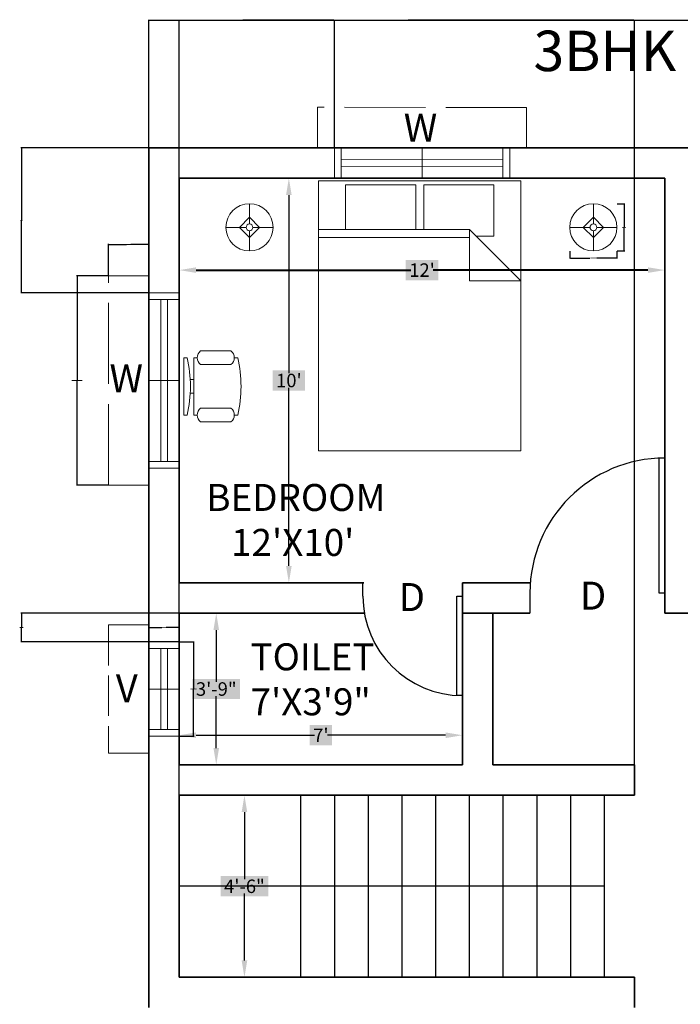
# Model space of a CAD drawing. Units: inches. Extents: x -128 to 854, y -395 to 398.
# Tile 35 of 61: x -88 to 107, y 95 to 387. Entities that reach past the tile are written whole.
import ezdxf

# ---------------------------------------------------------------- set-up
doc = ezdxf.new("R2010")
doc.units = ezdxf.units.IN
doc.header["$MEASUREMENT"] = 0
doc.linetypes.add('ACAD_ISO02W100', pattern=[15, 12, -3])
for name, color, linetype, lineweight in [('A-ANNO-DIMS', 2, 'Continuous', 18), ('A-ANNO-TEXT', 2, 'Continuous', 18), ('A-ANNO-TITL', 7, 'Continuous', 25), ('A-AREA-IDEN', 1, 'Continuous', 18), ('A-DOOR', 4, 'Continuous', 25), ('A-FLOR-STRS', 7, 'Continuous', 25), ('A-FURN', 8, 'Continuous', 18), ('A-GLAZ', 220, 'Continuous', 18), ('A-GLAZ-OVHD', 220, 'ACAD_ISO02W100', 13), ('A-WALL', 4, 'Continuous', 35)]:
    doc.layers.add(name, color=color, linetype=linetype, lineweight=lineweight)
doc.styles.get("Standard").update_dxf_attribs({"font": 'arial.ttf'})
doc.dimstyles.get("Standard").update_dxf_attribs({"dimtxt": 0.18, "dimasz": 0.18, "dimexe": 0.18, "dimexo": 0.0625, "dimgap": 0.09, "dimtad": 0, "dimtih": 1, "dimtoh": 1, "dimdec": 1, "dimzin": 0, "dimdsep": 46, "dimlunit": 4, "dimtxsty": 'Standard', "dimcen": 0.09, "dimclrd": 1, "dimclre": 2, "dimclrt": 6, "dimadec": 0, "dimazin": 0, "dimtfac": 1, "dimtdec": 1, "dimtofl": 0, "dimtmove": 0, "dimatfit": 3, "dimfxl": 1, "dimtfill": 2, "dimtfillclr": 3, "dimtolj": 1, "dimtzin": 0, "dimarcsym": 0})

# ---------------------------------------------------------------- blocks, each defined once
blk = doc.blocks.new('*U6')
for p, q in [((0, 0), (0, -6)), ((-40, 0), (-40, -6))]:
    blk.add_line(p, q)
blk.add_lwpolyline([(0, 0), (0, 40), (-1.75, 40), (-1.75, 0)], close=True)
blk.add_arc((0, 0), 40, 90, 180)
blk = doc.blocks.new('*U5')
for p, q in [((-750, 0), (-750, 100)), ((0, 0), (0, 100))]:
    blk.add_line(p, q)
blk.add_lwpolyline([(0, 0), (0, -750), (-43.75, -750), (-43.75, 0)], close=True)
blk.add_arc((0, 0), 750, 180, 270)
blk = doc.blocks.new('Chair - Desk')
for p, q in [((-8.5, 0), (-8.5, -1)), ((-8.5, 0), (8.5, 0)), ((8.5, 0), (8.5, -1)), ((-2, -3), (-2, -1.9355)), ((2, -1.9576), (2, -3)), ((-10.5, -5), (-10.5, -14)), ((-8.5, -3), (-8.5, -4)), ((-8.5, -3), (8.5, -3)), ((-6.5, -14), (-6.5, -5)), ((6.5, -5), (6.5, -14)), ((8.5, -3), (8.5, -4)), ((10.5, -14), (10.5, -5)), ((-8.5, -15), (-8.5, -16)), ((8.5, -15), (8.5, -16))]:
    blk.add_line(p, q)
for centre, radius, start, end in [((0, 34.625), 36.625, 256.5803, 283.4197), ((-8.5, -6.5), 2.5, 36.8699, 143.1301), ((8.5, -6.5), 2.5, 36.8699, 143.1301), ((-8.5, -12.5), 2.5, 216.8699, 323.1301), ((8.5, -12.5), 2.5, 216.8699, 323.1301), ((0, 19.625), 36.625, 256.5803, 283.4197)]:
    blk.add_arc(centre, radius, start, end)
blk = doc.blocks.new('Bed - Queen')
for p, q in [((0, -80.00003), (0, 0)), ((0, 0), (59.99999, 0)), ((59.99999, 0), (59.99999, -80.00003)), ((7.99999, -1.2), (28.79998, -1.2)), ((7.99999, -14.4), (7.99999, -1.2)), ((28.79998, -1.2), (28.79998, -14.4)), ((31.19999, -1.2), (51.99999, -1.2)), ((31.19999, -14.4), (31.19999, -1.2)), ((51.99999, -1.2), (51.99999, -16.4)), ((0, -14.4), (44.8, -14.4)), ((59.99999, -29.6), (44.8, -14.4)), ((44.8, -14.4), (44.8, -29.6)), ((44.8, -16.8), (0, -16.8)), ((51.99999, -16.4), (46.79936, -16.4)), ((44.8, -29.6), (59.99999, -29.6)), ((59.99999, -80.00003), (0, -80.00003))]:
    blk.add_line(p, q)
blk = doc.blocks.new('Lamp - Table')
for p, q in [((0, 7), (0, 1)), ((0, 3), (-3, 0)), ((3, 0), (0, 3)), ((-1, 0), (-7, 0)), ((-3, 0), (0, -3)), ((0, -3), (3, 0)), ((1, 0), (7, 0)), ((0, -1), (0, -7))]:
    blk.add_line(p, q)
for radius in [7, 1]:
    blk.add_circle((0, 0), radius)
blk = doc.blocks.new('*D46')
at = {"layer": 'A-ANNO-DIMS', "color": 0, "lineweight": -2, "transparency": 16777216}
for p, q in [((-41.13, 165.8), (-41.13, 174.71)), ((-36.13, 174.53), (-1.04, 174.53)), ((37.87, 174.53), (2.79, 174.53)), ((42.87, 165.8), (42.87, 174.71))]:
    blk.add_line(p, q, dxfattribs=at)
at = {"layer": 'A-ANNO-DIMS', "color": 0, "transparency": 16777216}
for points in [[(-36.13, 175.37), (-36.13, 173.7), (-41.13, 174.53)], [(37.87, 175.37), (37.87, 173.7), (42.87, 174.53)]]:
    blk.add_solid(points, dxfattribs=at)
at = {"layer": 'Defpoints', "color": 0, "transparency": 16777216}
for p in [(42.87, 174.53), (-41.13, 165.74), (42.87, 165.74)]:
    blk.add_point(p, dxfattribs=at)
at = {"layer": 'A-ANNO-DIMS', "color": 0, "transparency": 16777216, "insert": (0.87, 174.53), "char_height": 4, "attachment_point": 5, "bg_fill": 1, "box_fill_scale": 1.25, "bg_fill_color": 3, "bg_fill_transparency": 0}
blk.add_mtext("\\A1;7'", dxfattribs=at)
blk = doc.blocks.new('*D47')
at = {"layer": 'A-ANNO-DIMS', "color": 0, "lineweight": -2, "transparency": 16777216}
for p, q in [((-41.06, 210.74), (-29.98, 210.74)), ((-30.16, 205.74), (-30.16, 190.37)), ((-30.16, 170.74), (-30.16, 186.11)), ((-41.06, 165.74), (-29.98, 165.74))]:
    blk.add_line(p, q, dxfattribs=at)
at = {"layer": 'A-ANNO-DIMS', "color": 0, "transparency": 16777216}
for points in [[(-31, 205.74), (-29.33, 205.74), (-30.16, 210.74)], [(-31, 170.74), (-29.33, 170.74), (-30.16, 165.74)]]:
    blk.add_solid(points, dxfattribs=at)
at = {"layer": 'Defpoints', "color": 0, "transparency": 16777216}
for p in [(-41.13, 210.74), (-41.13, 165.74), (-30.16, 165.74)]:
    blk.add_point(p, dxfattribs=at)
at = {"layer": 'A-ANNO-DIMS', "color": 0, "transparency": 16777216, "insert": (-30.16, 188.24), "char_height": 4, "attachment_point": 5, "bg_fill": 1, "box_fill_scale": 1.25, "bg_fill_color": 3, "bg_fill_transparency": 0}
blk.add_mtext('\\A1;3\'-9"', dxfattribs=at)
blk = doc.blocks.new('*D48')
at = {"layer": 'A-ANNO-DIMS', "color": 0, "lineweight": -2, "transparency": 16777216}
for p, q in [((-41.13, 339.68), (-41.13, 312.3)), ((102.87, 339.68), (102.87, 312.3))]:
    blk.add_line(p, q, dxfattribs=at)
at = {"layer": 'A-ANNO-DIMS', "color": 0, "lineweight": 40, "transparency": 16777216}
for p, q in [((-36.13, 312.48), (27.58, 312.48)), ((97.87, 312.48), (34.17, 312.48))]:
    blk.add_line(p, q, dxfattribs=at)
at = {"layer": 'A-ANNO-DIMS', "color": 0, "transparency": 16777216}
for points in [[(-36.13, 313.31), (-36.13, 311.65), (-41.13, 312.48)], [(97.87, 313.31), (97.87, 311.65), (102.87, 312.48)]]:
    blk.add_solid(points, dxfattribs=at)
at = {"layer": 'Defpoints', "color": 0, "transparency": 16777216}
for p in [(-41.13, 339.74), (102.87, 339.74), (102.87, 312.48)]:
    blk.add_point(p, dxfattribs=at)
at = {"layer": 'A-ANNO-DIMS', "color": 0, "transparency": 16777216, "insert": (30.87, 312.48), "char_height": 4, "attachment_point": 5, "bg_fill": 1, "box_fill_scale": 1.25, "bg_fill_color": 3, "bg_fill_transparency": 0}
blk.add_mtext("\\A1;12'", dxfattribs=at)
blk = doc.blocks.new('*D49')
at = {"layer": 'A-ANNO-DIMS', "color": 0, "lineweight": -2, "transparency": 16777216}
for p, q in [((-41.06, 339.74), (-8.45, 339.74)), ((-8.63, 334.74), (-8.63, 281.87)), ((-8.63, 224.74), (-8.63, 277.61)), ((-41.06, 219.74), (-8.45, 219.74))]:
    blk.add_line(p, q, dxfattribs=at)
at = {"layer": 'A-ANNO-DIMS', "color": 0, "transparency": 16777216}
for points in [[(-9.46, 334.74), (-7.8, 334.74), (-8.63, 339.74)], [(-9.46, 224.74), (-7.8, 224.74), (-8.63, 219.74)]]:
    blk.add_solid(points, dxfattribs=at)
at = {"layer": 'Defpoints', "color": 0, "transparency": 16777216}
for p in [(-41.13, 339.74), (-8.63, 339.74), (-41.13, 219.74)]:
    blk.add_point(p, dxfattribs=at)
at = {"layer": 'A-ANNO-DIMS', "color": 0, "transparency": 16777216, "insert": (-8.63, 279.74), "char_height": 4, "attachment_point": 5, "bg_fill": 1, "box_fill_scale": 1.25, "bg_fill_color": 3, "bg_fill_transparency": 0}
blk.add_mtext("\\A1;10'", dxfattribs=at)
blk = doc.blocks.new('*D54')
at = {"layer": 'A-ANNO-DIMS', "color": 0, "lineweight": -2, "transparency": 16777216}
for p, q in [((-41.06, 156.74), (-21.62, 156.74)), ((-21.8, 151.74), (-21.8, 131.87)), ((-21.8, 107.74), (-21.8, 127.61)), ((-41.06, 102.74), (-21.62, 102.74))]:
    blk.add_line(p, q, dxfattribs=at)
at = {"layer": 'A-ANNO-DIMS', "color": 0, "transparency": 16777216}
for points in [[(-22.63, 151.74), (-20.97, 151.74), (-21.8, 156.74)], [(-22.63, 107.74), (-20.97, 107.74), (-21.8, 102.74)]]:
    blk.add_solid(points, dxfattribs=at)
at = {"layer": 'Defpoints', "color": 0, "transparency": 16777216}
for p in [(-41.13, 156.74), (-21.8, 156.74), (-41.13, 102.74)]:
    blk.add_point(p, dxfattribs=at)
at = {"layer": 'A-ANNO-DIMS', "color": 0, "transparency": 16777216, "insert": (-21.8, 129.74), "char_height": 4, "attachment_point": 5, "bg_fill": 1, "box_fill_scale": 1.25, "bg_fill_color": 3, "bg_fill_transparency": 0}
blk.add_mtext('\\A1;4\'-6"', dxfattribs=at)
blk = doc.blocks.new('WIN-48IN')
for p, q in [((9, 52), (0, 52)), ((9, 50), (0, 50)), ((3.5, 50), (3.5, 2)), ((5.5, 50), (5.5, 2)), ((9, 26), (0, 26)), ((9, 2), (0, 2)), ((9, 0), (0, 0))]:
    blk.add_line(p, q)
blk = doc.blocks.new('SHADE-48IN')
at = {"ltscale": 2}
for p, q in [((12, 62), (0, 62)), ((0, 0), (0, 62)), ((12, 57), (12, 62)), ((12, 5), (12, 0)), ((12, 0), (0, 0))]:
    blk.add_line(p, q, dxfattribs=at)
blk = doc.blocks.new('VENT-24IN')
for p, q in [((0, 0), (0, 9)), ((2, 0), (2, 9)), ((14, 0), (14, 9)), ((26, 0), (26, 9)), ((28, 0), (28, 9)), ((2, 5.5), (26, 5.5)), ((2, 3.5), (26, 3.5))]:
    blk.add_line(p, q)
blk = doc.blocks.new('SHADE-24IN')
for p, q in [((0, 0), (0, 12)), ((38, 12), (0, 12)), ((38, 0), (38, 12)), ((5, 0), (0, 0)), ((33, 0), (38, 0))]:
    blk.add_line(p, q)
blk = doc.blocks.new('*D73')
at = {"layer": 'A-ANNO-DIMS', "color": 2, "lineweight": -2, "transparency": 16777216}
for p, q in [((-62.19, 310.74), (-71.61, 310.74)), ((-62.19, 248.74), (-71.61, 248.74))]:
    blk.add_line(p, q, dxfattribs=at)
at = {"layer": 'A-ANNO-DIMS', "color": 1, "lineweight": -2, "transparency": 16777216}
for p, q in [((-71.43, 310.56), (-71.43, 279.92)), ((-71.43, 248.92), (-71.43, 279.56))]:
    blk.add_line(p, q, dxfattribs=at)
at = {"layer": 'A-ANNO-DIMS', "color": 1, "transparency": 16777216}
for points in [[(-71.46, 310.56), (-71.4, 310.56), (-71.43, 310.74)], [(-71.46, 248.92), (-71.4, 248.92), (-71.43, 248.74)]]:
    blk.add_solid(points, dxfattribs=at)
at = {"layer": 'Defpoints', "color": 0, "transparency": 16777216}
for p in [(-71.43, 310.74), (-62.13, 310.74), (-62.13, 248.74)]:
    blk.add_point(p, dxfattribs=at)
at = {"layer": 'A-ANNO-DIMS', "color": 6, "transparency": 16777216, "insert": (-71.43, 279.74), "char_height": 0.18, "attachment_point": 5, "bg_fill": 1, "box_fill_scale": 1.25, "bg_fill_color": 3, "bg_fill_transparency": 0}
blk.add_mtext('\\A1;WINDOW SHADE 5\'-2" TYP.', dxfattribs=at)
blk = doc.blocks.new('*D74')
at = {"layer": 'A-ANNO-DIMS', "color": 2, "lineweight": -2, "transparency": 16777216}
for p, q in [((-62.13, 310.8), (-62.13, 320.22)), ((-50.13, 310.8), (-50.13, 320.22))]:
    blk.add_line(p, q, dxfattribs=at)
at = {"layer": 'A-ANNO-DIMS', "color": 1, "lineweight": -2, "transparency": 16777216}
for p, q in [((-61.95, 320.04), (-56.76, 320.04)), ((-50.31, 320.04), (-55.5, 320.04))]:
    blk.add_line(p, q, dxfattribs=at)
at = {"layer": 'A-ANNO-DIMS', "color": 1, "transparency": 16777216}
for points in [[(-61.95, 320.07), (-61.95, 320.01), (-62.13, 320.04)], [(-50.31, 320.07), (-50.31, 320.01), (-50.13, 320.04)]]:
    blk.add_solid(points, dxfattribs=at)
at = {"layer": 'Defpoints', "color": 0, "transparency": 16777216}
for p in [(-50.13, 320.04), (-62.13, 310.74), (-50.13, 310.74)]:
    blk.add_point(p, dxfattribs=at)
at = {"layer": 'A-ANNO-DIMS', "color": 6, "transparency": 16777216, "insert": (-56.13, 320.04), "char_height": 0.18, "attachment_point": 5, "bg_fill": 1, "box_fill_scale": 1.25, "bg_fill_color": 3, "bg_fill_transparency": 0}
blk.add_mtext('\\A1;1\'-0" TYP.', dxfattribs=at)
blk = doc.blocks.new('*D75')
at = {"layer": 'A-ANNO-DIMS', "color": 2, "lineweight": -2, "transparency": 16777216}
for p, q in [((74.69, 318.1), (74.69, 315.88)), ((88.69, 318.1), (88.69, 315.88))]:
    blk.add_line(p, q, dxfattribs=at)
at = {"layer": 'A-ANNO-DIMS', "color": 1, "lineweight": -2, "transparency": 16777216}
for p, q in [((74.87, 316.06), (80.68, 316.06)), ((88.51, 316.06), (82.71, 316.06))]:
    blk.add_line(p, q, dxfattribs=at)
at = {"layer": 'A-ANNO-DIMS', "color": 1, "transparency": 16777216}
for points in [[(74.87, 316.09), (74.87, 316.03), (74.69, 316.06)], [(88.51, 316.09), (88.51, 316.03), (88.69, 316.06)]]:
    blk.add_solid(points, dxfattribs=at)
at = {"layer": 'Defpoints', "color": 0, "transparency": 16777216}
for p in [(74.69, 318.16), (88.69, 318.16), (88.69, 316.06)]:
    blk.add_point(p, dxfattribs=at)
at = {"layer": 'A-ANNO-DIMS', "color": 6, "transparency": 16777216, "insert": (81.69, 316.06), "char_height": 0.18, "attachment_point": 5, "bg_fill": 1, "box_fill_scale": 1.25, "bg_fill_color": 3, "bg_fill_transparency": 0}
blk.add_mtext('\\A1;LAMP 1\'-2" TYP.', dxfattribs=at)
blk = doc.blocks.new('*D76')
at = {"layer": 'A-ANNO-DIMS', "color": 2, "lineweight": -2, "transparency": 16777216}
for p, q in [((88.76, 332.16), (90.97, 332.16)), ((88.76, 318.16), (90.97, 318.16))]:
    blk.add_line(p, q, dxfattribs=at)
at = {"layer": 'A-ANNO-DIMS', "color": 1, "lineweight": -2, "transparency": 16777216}
for p, q in [((90.79, 331.98), (90.79, 325.34)), ((90.79, 318.34), (90.79, 324.98))]:
    blk.add_line(p, q, dxfattribs=at)
at = {"layer": 'A-ANNO-DIMS', "color": 1, "transparency": 16777216}
for points in [[(90.76, 331.98), (90.82, 331.98), (90.79, 332.16)], [(90.76, 318.34), (90.82, 318.34), (90.79, 318.16)]]:
    blk.add_solid(points, dxfattribs=at)
at = {"layer": 'Defpoints', "color": 0, "transparency": 16777216}
for p in [(88.69, 332.16), (90.79, 332.16), (88.69, 318.16)]:
    blk.add_point(p, dxfattribs=at)
at = {"layer": 'A-ANNO-DIMS', "color": 6, "transparency": 16777216, "insert": (90.79, 325.16), "char_height": 0.18, "attachment_point": 5, "bg_fill": 1, "box_fill_scale": 1.25, "bg_fill_color": 3, "bg_fill_transparency": 0}
blk.add_mtext('\\A1;1\'-2" TYP.', dxfattribs=at)
blk = doc.blocks.new('*D79')
at = {"layer": 'A-ANNO-DIMS', "color": 2, "lineweight": -2, "transparency": 16777216}
for p, q in [((-41.06, 202.24), (-36.75, 202.24)), ((-41.06, 174.24), (-36.75, 174.24))]:
    blk.add_line(p, q, dxfattribs=at)
at = {"layer": 'A-ANNO-DIMS', "color": 1, "lineweight": -2, "transparency": 16777216}
for p, q in [((-36.93, 202.06), (-36.93, 188.42)), ((-36.93, 174.42), (-36.93, 188.06))]:
    blk.add_line(p, q, dxfattribs=at)
at = {"layer": 'A-ANNO-DIMS', "color": 1, "transparency": 16777216}
for points in [[(-36.96, 202.06), (-36.9, 202.06), (-36.93, 202.24)], [(-36.96, 174.42), (-36.9, 174.42), (-36.93, 174.24)]]:
    blk.add_solid(points, dxfattribs=at)
at = {"layer": 'Defpoints', "color": 0, "transparency": 16777216}
for p in [(-41.13, 202.24), (-41.13, 174.24), (-36.93, 174.24)]:
    blk.add_point(p, dxfattribs=at)
at = {"layer": 'A-ANNO-DIMS', "color": 6, "transparency": 16777216, "insert": (-36.93, 188.24), "char_height": 0.18, "attachment_point": 5, "bg_fill": 1, "box_fill_scale": 1.25, "bg_fill_color": 3, "bg_fill_transparency": 0}
blk.add_mtext('\\A1;VENT 2\'-4" TYP.', dxfattribs=at)
blk = doc.blocks.new('*D80')
at = {"layer": 'A-ANNO-DIMS', "color": 2, "lineweight": -2, "transparency": 16777216}
for p, q in [((-50.13, 202.3), (-50.13, 206.62)), ((-41.13, 202.3), (-41.13, 206.62))]:
    blk.add_line(p, q, dxfattribs=at)
at = {"layer": 'A-ANNO-DIMS', "color": 1, "lineweight": -2, "transparency": 16777216}
for p, q in [((-49.95, 206.44), (-46.27, 206.44)), ((-41.31, 206.44), (-44.99, 206.44))]:
    blk.add_line(p, q, dxfattribs=at)
at = {"layer": 'A-ANNO-DIMS', "color": 1, "transparency": 16777216}
for points in [[(-49.95, 206.47), (-49.95, 206.41), (-50.13, 206.44)], [(-41.31, 206.47), (-41.31, 206.41), (-41.13, 206.44)]]:
    blk.add_solid(points, dxfattribs=at)
at = {"layer": 'Defpoints', "color": 0, "transparency": 16777216}
for p in [(-41.13, 206.44), (-50.13, 202.24), (-41.13, 202.24)]:
    blk.add_point(p, dxfattribs=at)
at = {"layer": 'A-ANNO-DIMS', "color": 6, "transparency": 16777216, "insert": (-45.63, 206.44), "char_height": 0.18, "attachment_point": 5, "bg_fill": 1, "box_fill_scale": 1.25, "bg_fill_color": 3, "bg_fill_transparency": 0}
blk.add_mtext('\\A1;0\'-9" TYP.', dxfattribs=at)
blk = doc.blocks.new('*D97')
at = {"layer": 'A-ANNO-DIMS', "color": 2, "lineweight": -2, "transparency": 16777216}
for p, q in [((-50.13, 348.8), (-50.13, 386.74)), ((313.87, 348.8), (313.87, 386.74))]:
    blk.add_line(p, q, dxfattribs=at)
at = {"layer": 'A-ANNO-DIMS', "color": 1, "lineweight": -2, "transparency": 16777216}
for p, q in [((-49.95, 386.56), (131.47, 386.56)), ((313.69, 386.56), (132.27, 386.56))]:
    blk.add_line(p, q, dxfattribs=at)
at = {"layer": 'A-ANNO-DIMS', "color": 1, "transparency": 16777216}
for points in [[(-49.95, 386.59), (-49.95, 386.53), (-50.13, 386.56)], [(313.69, 386.59), (313.69, 386.53), (313.87, 386.56)]]:
    blk.add_solid(points, dxfattribs=at)
at = {"layer": 'Defpoints', "color": 0, "transparency": 16777216}
for p in [(313.87, 386.56), (-50.13, 348.74), (313.87, 348.74)]:
    blk.add_point(p, dxfattribs=at)
at = {"layer": 'A-ANNO-DIMS', "color": 6, "transparency": 16777216, "insert": (131.87, 386.56), "char_height": 0.18, "attachment_point": 5, "bg_fill": 1, "box_fill_scale": 1.25, "bg_fill_color": 3, "bg_fill_transparency": 0}
blk.add_mtext('\\A1;30\'-4"', dxfattribs=at)
blk = doc.blocks.new('*D103')
at = {"layer": 'A-ANNO-DIMS', "color": 2, "lineweight": -2, "transparency": 16777216}
for p, q in [((-41.13, 156.8), (-41.13, 386.74)), ((93.87, 156.8), (93.87, 386.74))]:
    blk.add_line(p, q, dxfattribs=at)
at = {"layer": 'A-ANNO-DIMS', "color": 1, "lineweight": -2, "transparency": 16777216}
for p, q in [((-40.95, 386.56), (25.98, 386.56)), ((93.69, 386.56), (26.76, 386.56))]:
    blk.add_line(p, q, dxfattribs=at)
at = {"layer": 'A-ANNO-DIMS', "color": 1, "transparency": 16777216}
for points in [[(-40.95, 386.59), (-40.95, 386.53), (-41.13, 386.56)], [(93.69, 386.59), (93.69, 386.53), (93.87, 386.56)]]:
    blk.add_solid(points, dxfattribs=at)
at = {"layer": 'Defpoints', "color": 0, "transparency": 16777216}
for p in [(93.87, 386.56), (-41.13, 156.74), (93.87, 156.74)]:
    blk.add_point(p, dxfattribs=at)
at = {"layer": 'A-ANNO-DIMS', "color": 6, "transparency": 16777216, "insert": (26.37, 386.56), "char_height": 0.18, "attachment_point": 5, "bg_fill": 1, "box_fill_scale": 1.25, "bg_fill_color": 3, "bg_fill_transparency": 0}
blk.add_mtext('\\A1;11\'-3"', dxfattribs=at)
blk = doc.blocks.new('*D104')
at = {"layer": 'A-ANNO-DIMS', "color": 2, "lineweight": -2, "transparency": 16777216}
for p, q in [((-50.13, 348.8), (-50.13, 386.74)), ((4.88, 348.83), (4.88, 386.74))]:
    blk.add_line(p, q, dxfattribs=at)
at = {"layer": 'A-ANNO-DIMS', "color": 1, "lineweight": -2, "transparency": 16777216}
for p, q in [((-49.95, 386.56), (-22.96, 386.56)), ((4.7, 386.56), (-22.29, 386.56))]:
    blk.add_line(p, q, dxfattribs=at)
at = {"layer": 'A-ANNO-DIMS', "color": 1, "transparency": 16777216}
for points in [[(-49.95, 386.59), (-49.95, 386.53), (-50.13, 386.56)], [(4.7, 386.59), (4.7, 386.53), (4.88, 386.56)]]:
    blk.add_solid(points, dxfattribs=at)
at = {"layer": 'Defpoints', "color": 0, "transparency": 16777216}
for p in [(4.88, 386.56), (-50.13, 348.74), (4.88, 348.76)]:
    blk.add_point(p, dxfattribs=at)
at = {"layer": 'A-ANNO-DIMS', "color": 6, "transparency": 16777216, "insert": (-22.62, 386.56), "char_height": 0.18, "attachment_point": 5, "bg_fill": 1, "box_fill_scale": 1.25, "bg_fill_color": 3, "bg_fill_transparency": 0}
blk.add_mtext('\\A1;4\'-7"', dxfattribs=at)
blk = doc.blocks.new('*D107')
at = {"layer": 'A-ANNO-DIMS', "color": 2, "lineweight": -2, "transparency": 16777216}
for p, q in [((-50.19, 348.74), (-88.11, 348.74)), ((-50.19, 305.74), (-88.11, 305.74))]:
    blk.add_line(p, q, dxfattribs=at)
at = {"layer": 'A-ANNO-DIMS', "color": 1, "lineweight": -2, "transparency": 16777216}
for p, q in [((-87.93, 348.56), (-87.93, 327.42)), ((-87.93, 305.92), (-87.93, 327.06))]:
    blk.add_line(p, q, dxfattribs=at)
at = {"layer": 'A-ANNO-DIMS', "color": 1, "transparency": 16777216}
for points in [[(-87.96, 348.56), (-87.9, 348.56), (-87.93, 348.74)], [(-87.96, 305.92), (-87.9, 305.92), (-87.93, 305.74)]]:
    blk.add_solid(points, dxfattribs=at)
at = {"layer": 'Defpoints', "color": 0, "transparency": 16777216}
for p in [(-50.13, 348.74), (-87.93, 305.74), (-50.13, 305.74)]:
    blk.add_point(p, dxfattribs=at)
at = {"layer": 'A-ANNO-DIMS', "color": 6, "transparency": 16777216, "insert": (-87.93, 327.24), "char_height": 0.18, "attachment_point": 5, "bg_fill": 1, "box_fill_scale": 1.25, "bg_fill_color": 3, "bg_fill_transparency": 0}
blk.add_mtext('\\A1;3\'-7"', dxfattribs=at)
blk = doc.blocks.new('*D108')
at = {"layer": 'A-ANNO-DIMS', "color": 2, "lineweight": -2, "transparency": 16777216}
for p, q in [((-41.19, 210.74), (-88.11, 210.74)), ((-41.19, 202.24), (-88.11, 202.24))]:
    blk.add_line(p, q, dxfattribs=at)
at = {"layer": 'A-ANNO-DIMS', "color": 1, "lineweight": -2, "transparency": 16777216}
for p, q in [((-87.93, 210.56), (-87.93, 206.67)), ((-87.93, 202.42), (-87.93, 206.31))]:
    blk.add_line(p, q, dxfattribs=at)
at = {"layer": 'A-ANNO-DIMS', "color": 1, "transparency": 16777216}
for points in [[(-87.96, 210.56), (-87.9, 210.56), (-87.93, 210.74)], [(-87.96, 202.42), (-87.9, 202.42), (-87.93, 202.24)]]:
    blk.add_solid(points, dxfattribs=at)
at = {"layer": 'Defpoints', "color": 0, "transparency": 16777216}
for p in [(-41.13, 210.74), (-87.93, 202.24), (-41.13, 202.24)]:
    blk.add_point(p, dxfattribs=at)
at = {"layer": 'A-ANNO-DIMS', "color": 6, "transparency": 16777216, "insert": (-87.93, 206.49), "char_height": 0.18, "attachment_point": 5, "bg_fill": 1, "box_fill_scale": 1.25, "bg_fill_color": 3, "bg_fill_transparency": 0}
blk.add_mtext('\\A1;0\'-8 1/2"', dxfattribs=at)

msp = doc.modelspace()

# ---------------------------------------------------------------- linework, layer by layer
at = {"layer": 'A-FLOR-STRS'}
for p, q in [((-5.13, 156.74), (-5.13, 102.74)), ((4.87, 156.74), (4.87, 102.74)), ((14.87, 156.74), (14.87, 102.74)), ((24.87, 156.74), (24.87, 102.74)), ((34.87, 156.74), (34.87, 102.74)), ((44.87, 156.74), (44.87, 102.74)), ((54.87, 156.74), (54.87, 102.74)), ((64.87, 156.74), (64.87, 102.74)), ((74.87, 156.74), (74.87, 102.74)), ((84.87, 156.74), (84.87, 102.74)), ((84.87, 129.74), (-41.13, 129.74))]:
    msp.add_line(p, q, dxfattribs=at)
at = {"layer": 'A-GLAZ-OVHD', "ltscale": 2}
for p, q in [((-0.12, 348.76), (-0.12, 360.76)), ((61.88, 360.72), (-0.12, 360.76)), ((61.88, 348.72), (61.88, 360.72)), ((4.88, 348.76), (-0.12, 348.76)), ((56.88, 348.72), (61.88, 348.72))]:
    msp.add_line(p, q, dxfattribs=at)
at = {"layer": 'A-WALL'}
for p, q in [((-50.13, 210.74), (-50.13, 348.74)), ((-50.13, 348.74), (111.87, 348.74)), ((-41.13, 339.74), (102.87, 339.74)), ((-41.13, 219.74), (-41.13, 339.74)), ((102.87, 339.74), (102.87, 210.74)), ((13.61, 219.74), (-41.13, 219.74)), ((42.87, 165.74), (42.87, 219.74)), ((62.99, 219.74), (42.87, 219.74)), ((-50.13, 210.74), (-50.13, 156.74)), ((-41.13, 210.74), (-41.13, 165.74)), ((13.78, 210.74), (-41.13, 210.74)), ((62.87, 210.74), (42.87, 210.74)), ((51.87, 165.74), (51.87, 210.74)), ((111.87, 210.74), (102.87, 210.74)), ((-41.13, 165.74), (42.87, 165.74)), ((51.87, 165.74), (93.87, 165.74)), ((93.87, 165.74), (93.87, 156.74)), ((-50.13, 156.74), (-50.13, 93.74)), ((-41.13, 156.74), (51.87, 156.74)), ((-41.13, 156.74), (-41.13, 102.74)), ((51.87, 156.74), (93.87, 156.74)), ((-41.13, 102.74), (51.87, 102.74)), ((51.87, 102.74), (93.87, 102.74)), ((93.87, 102.74), (93.87, 93.74))]:
    msp.add_line(p, q, dxfattribs=at)

# ---------------------------------------------------------------- block references
at = {"layer": 'A-DOOR'}
msp.add_blockref('*U6', (102.87, 216.74), dxfattribs=at)
at = {"layer": 'A-DOOR', "xscale": 0.0393700787401575, "yscale": 0.0393700787401575, "zscale": 0.0393700787401575}
msp.add_blockref('*U5', (42.87, 215.8), dxfattribs=at)
at = {"layer": 'A-FURN'}
for name, p in [('Bed - Queen', (0.18, 338.92)), ('Lamp - Table', (-20.3, 325.16)), ('Lamp - Table', (81.69, 325.16))]:
    msp.add_blockref(name, p, dxfattribs=at)
at = {"layer": 'A-FURN', "rotation": 90}
msp.add_blockref('Chair - Desk', (-39.81, 277.99), dxfattribs=at)
at = {"layer": 'A-GLAZ'}
for name, p, rotation in [('WIN-48IN', (56.87, 339.72), 89.95157271250135), ('VENT-24IN', (-50.13, 202.24), 269.9999999999995)]:
    msp.add_blockref(name, p, dxfattribs=dict(at, rotation=rotation))
msp.add_blockref('WIN-48IN', (-50.13, 253.74), dxfattribs=at)
at = {"layer": 'A-GLAZ-OVHD'}
msp.add_blockref('SHADE-48IN', (-62.13, 248.74), dxfattribs=at)
at = {"layer": 'A-GLAZ-OVHD', "rotation": 89.99999999999999}
msp.add_blockref('SHADE-24IN', (-50.13, 169.24), dxfattribs=at)

# ---------------------------------------------------------------- texts
at = {"layer": 'A-ANNO-TEXT'}
for s, p in [('W', (25.44, 350.57)), ('W', (-61.84, 276.24)), ('D', (23.96, 211.36)), ('D', (77.7, 211.77)), ('V', (-59.96, 184.32))]:
    msp.add_text(s, height=8.31, dxfattribs=at).set_placement(p)
at = {"layer": 'A-ANNO-TITL'}
msp.add_text('3BHK HOME PLAN', height=12, dxfattribs=at).set_placement((63.94, 371.49))
at = {"layer": 'A-AREA-IDEN', "char_height": 8, "attachment_point": 1}
for s, insert in [("BEDROOM\\P   12'X10'", (-33.09, 249.05)), ('TOILET\\P7\'X3\'9"', (-19.98, 201.79))]:
    msp.add_mtext_dynamic_manual_height_columns(s, width=99.0352, gutter_width=1, heights=[0], dxfattribs=dict(at, insert=insert))

# ---------------------------------------------------------------- dimensions: what is measured, and where the dimension line sits
at = {"layer": 'A-ANNO-DIMS'}
for base, p1, p2, override, picture, middle in [((313.87, 386.56), (-50.13, 348.74), (313.87, 348.74), {"dimdec": 1, "dimlfac": 1, "dimrnd": 0, "dimzin": 1, "dimdsep": 46, "dimlunit": 4, "dimfrac": 2}, '*D97', (131.87, 386.56)), ((4.88, 386.56), (-50.13, 348.74), (4.88, 348.76), {"dimdec": 1, "dimlfac": 1, "dimrnd": 0, "dimzin": 1, "dimdsep": 46, "dimlunit": 4, "dimfrac": 2}, '*D104', (-22.62, 386.56)), ((93.87, 386.56), (-41.13, 156.74), (93.87, 156.74), {"dimdec": 1, "dimlfac": 1, "dimrnd": 0, "dimzin": 1, "dimdsep": 46, "dimlunit": 4, "dimfrac": 2}, '*D103', (26.37, 386.56)), ((102.87, 312.48), (-41.13, 339.74), (102.87, 339.74), {"dimtxt": 4, "dimasz": 5, "dimclrd": 0, "dimclre": 0, "dimclrt": 0, "dimlwd": 40}, '*D48', (30.87, 312.48)), ((42.87, 174.53), (-41.13, 165.74), (42.87, 165.74), {"dimtxt": 4, "dimasz": 5, "dimclrd": 0, "dimclre": 0, "dimclrt": 0}, '*D46', (0.87, 174.53))]:
    dim = msp.add_linear_dim(base=base, p1=p1, p2=p2, dimstyle='Standard', override=override, dxfattribs=at)
    dim.commit()
    dim.dimension.update_dxf_attribs({"geometry": picture, "text_midpoint": middle})
for base, p1, p2, override, picture, middle in [((-87.93, 305.74), (-50.13, 348.74), (-50.13, 305.74), {"dimdec": 1, "dimlfac": 1, "dimrnd": 0, "dimzin": 1, "dimdsep": 46, "dimlunit": 4, "dimfrac": 2}, '*D107', (-87.93, 327.24)), ((-8.63, 339.74), (-41.13, 219.74), (-41.13, 339.74), {"dimtxt": 4, "dimasz": 5, "dimclrd": 0, "dimclre": 0, "dimclrt": 0}, '*D49', (-8.63, 279.74)), ((-87.93, 202.24), (-41.13, 210.74), (-41.13, 202.24), {"dimdec": 1, "dimlfac": 1, "dimrnd": 0, "dimzin": 1, "dimdsep": 46, "dimlunit": 4, "dimfrac": 2}, '*D108', (-87.93, 206.49)), ((-30.16, 165.74), (-41.13, 210.74), (-41.13, 165.74), {"dimtxt": 4, "dimasz": 5, "dimclrd": 0, "dimclre": 0, "dimclrt": 0}, '*D47', (-30.16, 188.24)), ((-21.8, 156.74), (-41.13, 102.74), (-41.13, 156.74), {"dimtxt": 4, "dimasz": 5, "dimclrd": 0, "dimclre": 0, "dimclrt": 0}, '*D54', (-21.8, 129.74))]:
    dim = msp.add_linear_dim(base=base, p1=p1, p2=p2, angle=90, dimstyle='Standard', override=override, dxfattribs=at)
    dim.commit()
    dim.dimension.update_dxf_attribs({"geometry": picture, "text_midpoint": middle})
for base, p1, p2, angle, text, picture, middle in [((90.79, 332.16), (88.69, 318.16), (88.69, 332.16), 90, '<> TYP.', '*D76', (90.79, 325.16)), ((-71.43, 310.74), (-62.13, 248.74), (-62.13, 310.74), 90, 'WINDOW SHADE <> TYP.', '*D73', (-71.43, 279.74)), ((-36.93, 174.24), (-41.13, 202.24), (-41.13, 174.24), 270, 'VENT <> TYP.', '*D79', (-36.93, 188.24))]:
    dim = msp.add_linear_dim(base=base, p1=p1, p2=p2, angle=angle, text=text, dimstyle='Standard', override={"dimdec": 1, "dimlfac": 1, "dimrnd": 0, "dimzin": 1, "dimdsep": 46, "dimlunit": 4, "dimfrac": 2}, dxfattribs=at)
    dim.commit()
    dim.dimension.update_dxf_attribs({"geometry": picture, "text_midpoint": middle})
for base, p1, p2, text, picture, middle in [((-50.13, 320.04), (-62.13, 310.74), (-50.13, 310.74), '<> TYP.', '*D74', (-56.13, 320.04)), ((88.69, 316.06), (74.69, 318.16), (88.69, 318.16), 'LAMP <> TYP.', '*D75', (81.69, 316.06)), ((-41.13, 206.44), (-50.13, 202.24), (-41.13, 202.24), '<> TYP.', '*D80', (-45.63, 206.44))]:
    dim = msp.add_linear_dim(base=base, p1=p1, p2=p2, text=text, dimstyle='Standard', override={"dimdec": 1, "dimlfac": 1, "dimrnd": 0, "dimzin": 1, "dimdsep": 46, "dimlunit": 4, "dimfrac": 2}, dxfattribs=at)
    dim.commit()
    dim.dimension.update_dxf_attribs({"geometry": picture, "text_midpoint": middle})

doc.saveas('drawing.dxf')
